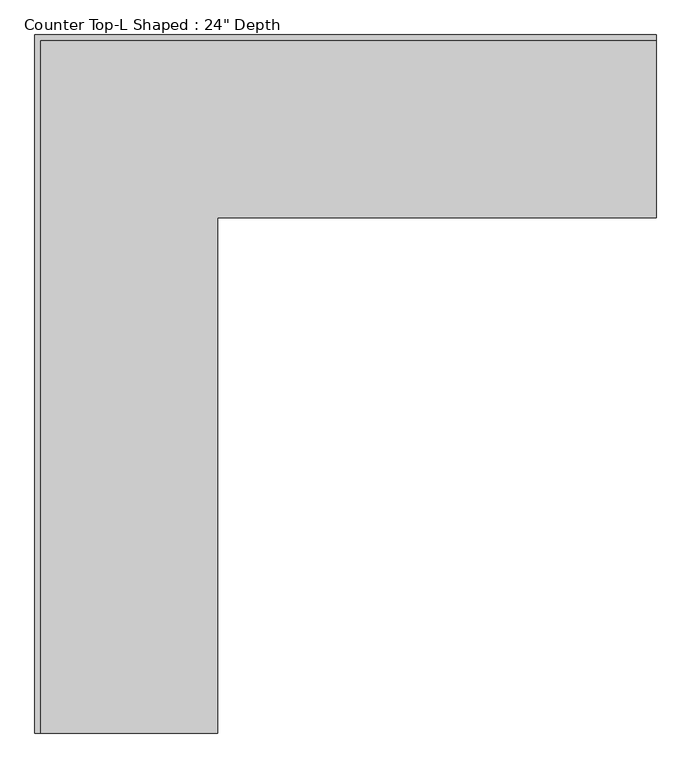
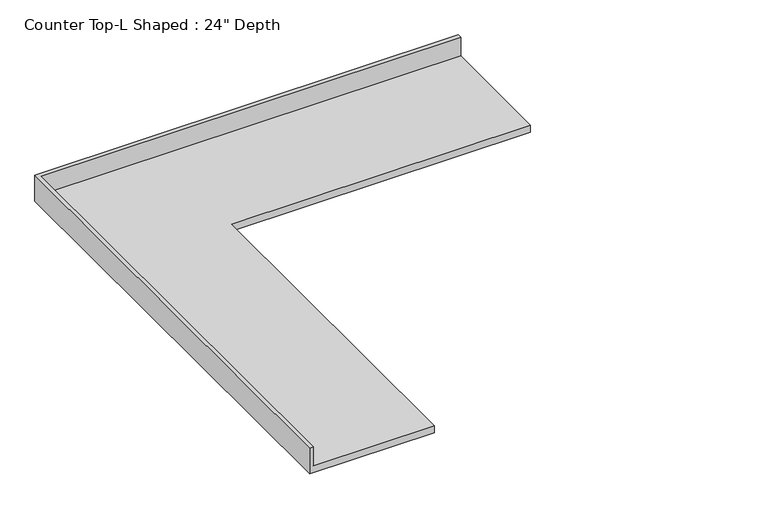
"""IFC4 building model written with IfcOpenShell, lengths in millimetres: furniture geometry."""

from ifc_helpers import new_model, si_unit, origin, place, context, project, spatial, faceted_brep, source, transform, mapped, element, save


def furniture_a71f50c7(model_context):
    return source(origin(), model_context, "Body", "Brep", [
        faceted_brep([(-565.4622951, -2424.7238313, 914.4), (-565.4622951, -635.0, 914.4), (958.5377049, -635.0, 914.4), (958.5377049, -19.05, 914.4), (-1181.4122951, -19.05, 914.4), (-1181.4122951, -2424.7238313, 914.4), (958.5377049, 0.0, 876.3), (958.5377049, -635.0, 876.3), (-565.4622951, -635.0, 876.3), (-565.4622951, -2424.7238313, 876.3), (-1200.4622951, -2424.7238313, 876.3), (-1200.4622951, 0.0, 876.3), (-1200.4622951, 0.0, 1016.0), (958.5377049, 0.0, 1016.0), (-1200.4622951, -2424.7238313, 1016.0), (-1181.4122951, -2424.7238313, 1016.0), (958.5377049, -19.05, 1016.0), (-1181.4122951, -19.05, 1016.0)], [[[0, 1, 2, 3, 4, 5]], [[6, 7, 8, 9, 10, 11]], [[6, 11, 12, 13]], [[11, 10, 14, 12]], [[14, 10, 9, 0, 5, 15]], [[1, 0, 9, 8]], [[2, 1, 8, 7]], [[7, 6, 13, 16, 3, 2]], [[12, 14, 15, 17, 16, 13]], [[3, 16, 17, 4]], [[17, 15, 5, 4]]]),
    ])


if __name__ == "__main__":
    model = new_model("IFC4")
    model_context = context("Model", 3, world=origin())
    ifc_project = project(units=[si_unit("LENGTHUNIT", "METRE", prefix="MILLI")], contexts=[model_context])
    site = spatial("IfcSite", under=ifc_project)
    building = spatial("IfcBuilding", under=site)
    placement = place(None, origin())
    furniture_shape = furniture_a71f50c7(model_context)
    element("IfcFurniture", 1, ObjectType="Counter Top-L Shaped : 24\" Depth", at=placement, inside=building, context=model_context, shape_type="MappedRepresentation", body=[
        mapped(furniture_shape, transform((0.0, 0.0, 0.0), x_axis=(1.0, 0.0, 0.0), y_axis=(0.0, 1.0, 0.0), z_axis=(0.0, 0.0, 1.0))),
    ])
    save(model, "model.ifc")

# Revit data of these elements
# Type "Counter Top-L Shaped : 24\" Depth"
#   Assembly Code = "C1030400"
#   Counter Thickness = 0' - 1 1/2"
#   Depth = 2' - 1"
#   Height = 3' - 0"
#   Length - Leg 1 [instance default] = 8' - 0"
#   Length - Leg 2 [instance default] = 6' - 0"
#   Counter Top Material = none
#   Default Elevation = 0
# Element 1 (IfcFurniture, "Counter Top-L Shaped : 24\" Depth")
#   Length - Leg 1 = 7' - 1"
#   Length - Leg 2 = 7' - 11.46157"
#   Materials on its faces: "Counter Top"
# Materials
#   "Counter Top": class "Wood", colour RGB 226 177 128, transparency 0
